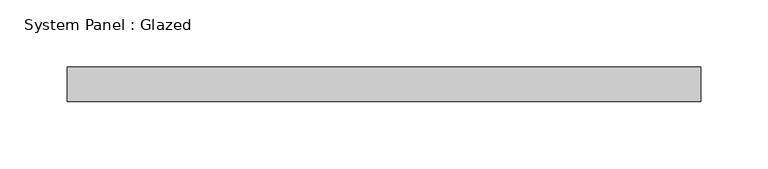
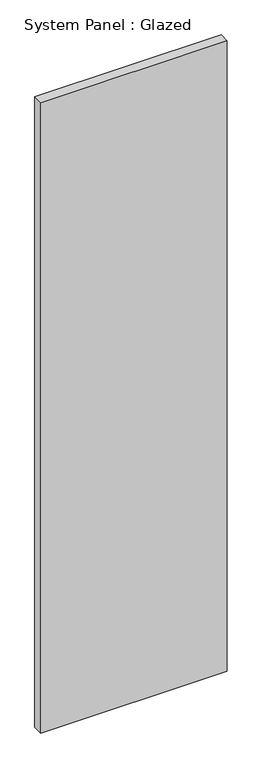
"""IFC4 building model written with IfcOpenShell, lengths in millimetres: plate geometry, System Panel : Glazed."""

from ifc_helpers import new_model, si_unit, origin, origin_with_axes, place, context, project, spatial, polyline, outline, extrude, source, transform, mapped, element, save


def system_panel_glazed_bef0ddaa(model_context):
    return source(origin(), model_context, "Body", "SweptSolid", [
        extrude(outline(polyline([(234.95, 19.05), (-234.95, 19.05), (-234.95, 44.45), (234.95, 44.45), (234.95, 19.05)])), origin_with_axes(), (0.0, 0.0, 1.0), 1678.4265918),
    ])


if __name__ == "__main__":
    model = new_model("IFC4")
    model_context = context("Model", 3, world=origin())
    ifc_project = project(units=[si_unit("LENGTHUNIT", "METRE", prefix="MILLI")], contexts=[model_context])
    site = spatial("IfcSite", under=ifc_project)
    building = spatial("IfcBuilding", under=site)
    placement = place(None, origin())
    system_panel_glazed_shape = system_panel_glazed_bef0ddaa(model_context)
    element("IfcPlate", 1, ObjectType="System Panel : Glazed", at=placement, inside=building, context=model_context, shape_type="MappedRepresentation", body=[
        mapped(system_panel_glazed_shape, transform((0.0, 0.0, 0.0), x_axis=(1.0, 0.0, 0.0), y_axis=(0.0, 1.0, 0.0), z_axis=(0.0, 0.0, 1.0))),
    ])
    save(model, "model.ifc")

# Revit data of these elements
# Type "System Panel : Glazed"
#   Construction Type Id = "GSP4R"
#   Analytic Construction = "1/8 in Pilkington single glazing"
#   Visual Light Transmittance = 0.9
#   Solar Heat Gain Coefficient = 0.86
#   Heat Transfer Coefficient (U) = 1.18115 BTU/(h·ft²·°F)
#   Define Thermal Properties by = 1
# Element 1 (IfcPlate, "System Panel : Glazed")
#   Materials on its faces: "Glass"
# Materials
#   "Glass": class "Glass", colour RGB 0 128 192, transparency 0.75, Description = "Soda Lime Glass", Cost = 0
